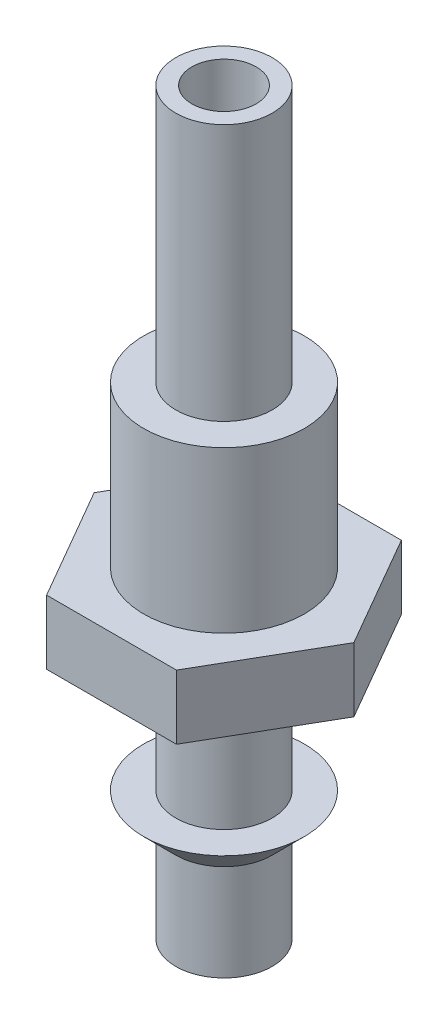
SolidWorks part; units mm, degrees
material "Plain Carbon Steel"
ref_plane "Front Plane" through (0, 0, 0) normal (0, 0, 1) x (1, 0, 0)
ref_plane "Top Plane" through (0, 0, 0) normal (0, 1, 0) x (1, 0, 0)
ref_plane "Right Plane" through (0, 0, 0) normal (1, 0, 0) x (0, 0, -1)
sketch "Lower Spigot Profile" plane through (0, 0, 0) normal (0, 0, 1) x (1, 0, 0)
  line L0 (0, 0) -> (0, -8)
  line L1 (0, -8) -> (1.5, -8)
  line L2 (1.5, -8) -> (1.5, -5)
  line L3 (1.5, -5) -> (2.5, -4)
  line L4 (2.5, -4) -> (1.5, -4)
  line L5 (1.5, -4) -> (1.5, 0)
  line L6 (1.5, 0) -> (0, 0)
  dimension "D1" = 8
  dimension "D2" = 3
  dimension "D3" = 1
  dimension "D4" = 1.5
  dimension "D5" = 2.5
revolve "Lower Spigot and Collar" add sketch "Lower Spigot Profile" angle 360 about L0
sketch "Hex Profile 7AF" plane through (0, 0, 0) normal (0, 1, 0) x (1, 0, 0)
  line L1 (4.0415, 0) -> (2.0207, 3.5)
  line L2 (2.0207, 3.5) -> (-2.0207, 3.5)
  line L3 (-2.0207, 3.5) -> (-4.0415, 0)
  line L4 (-4.0415, 0) -> (-2.0207, -3.5)
  line L5 (-2.0207, -3.5) -> (2.0207, -3.5)
  line L6 (2.0207, -3.5) -> (4.0415, 0)
  circle A0 centre (0, 0) radius 3.5 construction
  dimension "D1" = 7
extrude "Hex 7AF" add sketch "Hex Profile 7AF" along normal blind 2
sketch "Upper Pipe Profile" plane through (0, 0, 0) normal (0, 0, 1) x (1, 0, 0)
  line L0 (0, 2) -> (0, 15)
  line L1 (-2.0207, 2) -> (2.0207, 2) construction
  line L2 (0, 15) -> (1.5, 15)
  line L3 (1.5, 15) -> (1.5, 7)
  line L4 (1.5, 7) -> (2.5, 7)
  line L5 (2.5, 7) -> (2.5, 2)
  line L6 (-1.5, -8) -> (1.5, -8) construction
  line L7 (0, 2) -> (2.5, 2)
  dimension "D1" = 23
  dimension "D2" = 15
  dimension "D3" = 2.5
  dimension "D4" = 1.5
revolve "Upper Pipe" add sketch "Upper Pipe Profile" angle 360 about L0
sketch "Bore Profile Ø2" plane through (0, 15, 0) normal (0, 1, 0) x (1, 0, 0)
  circle A0 centre (0, 0) radius 1
  dimension "D1" = 2
extrude "Fuel Bore Ø2" cut sketch "Bore Profile Ø2" against normal through all
